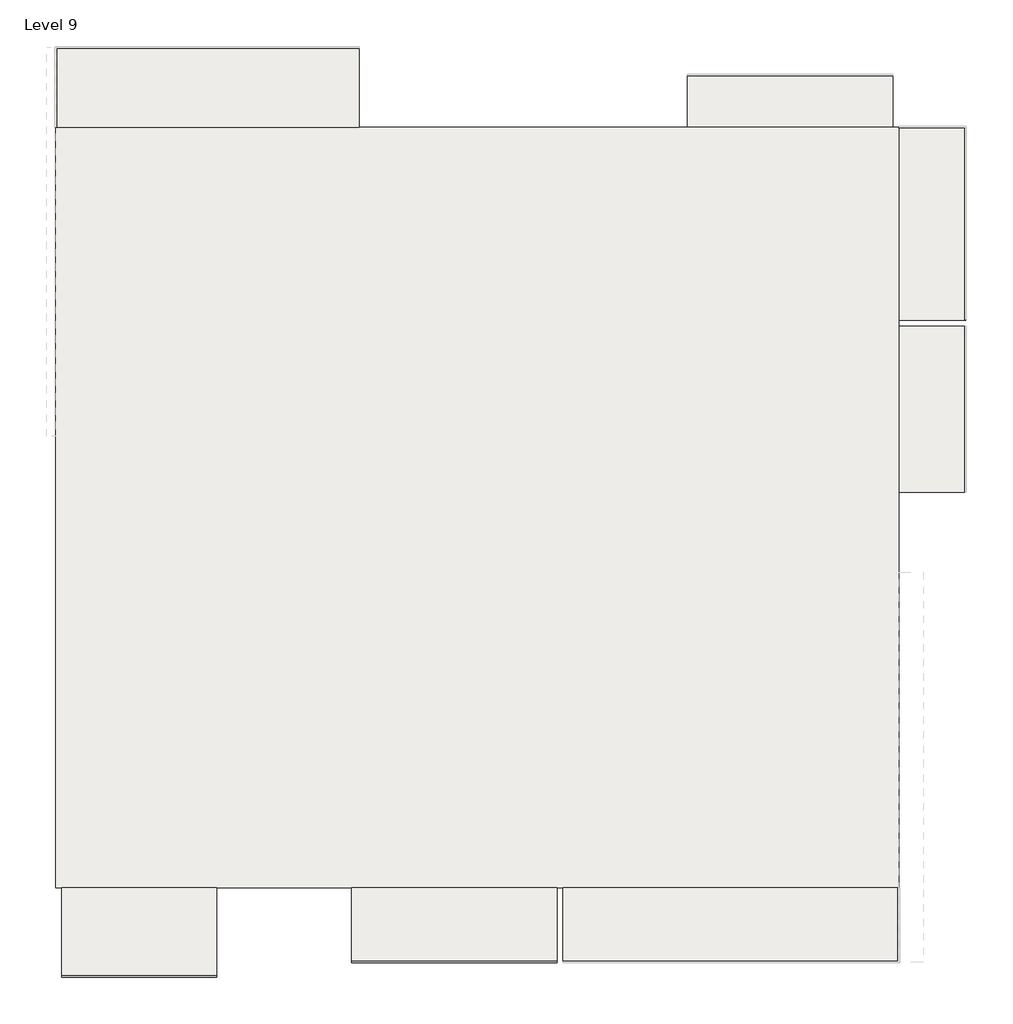
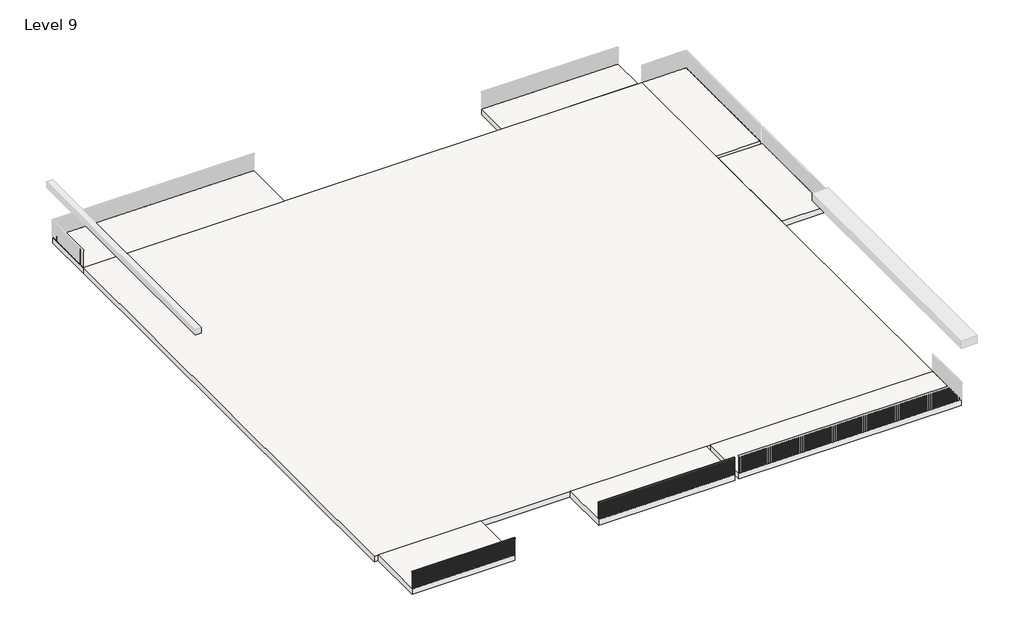
# One storey, part 1 of 5: 8 slabs, 2 railings.
"""IFC4 building model written with IfcOpenShell, lengths in millimetres."""

from ifc_helpers import new_model, si_unit, frame, origin, place, context, project, spatial, polyline, outline, extrude, element, save

model = new_model("IFC4")

# Units and contexts
model_context = context("Model", 3, world=origin())
ifc_project = project(units=[si_unit("LENGTHUNIT", "METRE", prefix="MILLI")], contexts=[model_context])

# Site, building, storey
site = spatial("IfcSite", under=ifc_project)
building = spatial("IfcBuilding", under=site)
storey = spatial("IfcBuildingStorey", under=building, Name="Level 9", Elevation=9448.8)

# Railings
placement = place(None, origin())
element("IfcRailing", 1, ObjectType="Handrail - Rectangular", at=placement, inside=storey, context=model_context, shape_type="SweptSolid", body=[
    extrude(outline(polyline([(-13630.2638778, -13399.9762475), (-13630.2638778, -13349.1762475), (-8499.4638778, -13349.1762475), (-8499.4638778, -13399.9762475), (-13630.2638778, -13399.9762475)])), frame((0.0, 0.0, 10312.4), z_axis=(0.0, 0.0, 1.0), x_axis=(1.0, 0.0, 0.0)), (0.0, 0.0, 1.0), 50.8),
    extrude(outline(polyline([(-8559.7888778, -13384.1012475), (-8559.7888778, -13365.0512475), (-8540.7388778, -13365.0512475), (-8540.7388778, -13384.1012475), (-8559.7888778, -13384.1012475)])), frame((0.0, 0.0, 9448.8), z_axis=(0.0, 0.0, 1.0), x_axis=(1.0, 0.0, 0.0)), (0.0, 0.0, 1.0), 863.6),
    extrude(outline(polyline([(-8661.3888778, -13384.1012475), (-8661.3888778, -13365.0512475), (-8642.3388778, -13365.0512475), (-8642.3388778, -13384.1012475), (-8661.3888778, -13384.1012475)])), frame((0.0, 0.0, 9448.8), z_axis=(0.0, 0.0, 1.0), x_axis=(1.0, 0.0, 0.0)), (0.0, 0.0, 1.0), 863.6),
    extrude(outline(polyline([(-8762.9888778, -13384.1012475), (-8762.9888778, -13365.0512475), (-8743.9388778, -13365.0512475), (-8743.9388778, -13384.1012475), (-8762.9888778, -13384.1012475)])), frame((0.0, 0.0, 9448.8), z_axis=(0.0, 0.0, 1.0), x_axis=(1.0, 0.0, 0.0)), (0.0, 0.0, 1.0), 863.6),
    extrude(outline(polyline([(-8864.5888778, -13384.1012475), (-8864.5888778, -13365.0512475), (-8845.5388778, -13365.0512475), (-8845.5388778, -13384.1012475), (-8864.5888778, -13384.1012475)])), frame((0.0, 0.0, 9448.8), z_axis=(0.0, 0.0, 1.0), x_axis=(1.0, 0.0, 0.0)), (0.0, 0.0, 1.0), 863.6),
    extrude(outline(polyline([(-8966.1888778, -13384.1012475), (-8966.1888778, -13365.0512475), (-8947.1388778, -13365.0512475), (-8947.1388778, -13384.1012475), (-8966.1888778, -13384.1012475)])), frame((0.0, 0.0, 9448.8), z_axis=(0.0, 0.0, 1.0), x_axis=(1.0, 0.0, 0.0)), (0.0, 0.0, 1.0), 863.6),
    extrude(outline(polyline([(-9067.7888778, -13384.1012475), (-9067.7888778, -13365.0512475), (-9048.7388778, -13365.0512475), (-9048.7388778, -13384.1012475), (-9067.7888778, -13384.1012475)])), frame((0.0, 0.0, 9448.8), z_axis=(0.0, 0.0, 1.0), x_axis=(1.0, 0.0, 0.0)), (0.0, 0.0, 1.0), 863.6),
    extrude(outline(polyline([(-9169.3888778, -13384.1012475), (-9169.3888778, -13365.0512475), (-9150.3388778, -13365.0512475), (-9150.3388778, -13384.1012475), (-9169.3888778, -13384.1012475)])), frame((0.0, 0.0, 9448.8), z_axis=(0.0, 0.0, 1.0), x_axis=(1.0, 0.0, 0.0)), (0.0, 0.0, 1.0), 863.6),
    extrude(outline(polyline([(-9270.9888778, -13384.1012475), (-9270.9888778, -13365.0512475), (-9251.9388778, -13365.0512475), (-9251.9388778, -13384.1012475), (-9270.9888778, -13384.1012475)])), frame((0.0, 0.0, 9448.8), z_axis=(0.0, 0.0, 1.0), x_axis=(1.0, 0.0, 0.0)), (0.0, 0.0, 1.0), 863.6),
    extrude(outline(polyline([(-9372.5888778, -13384.1012475), (-9372.5888778, -13365.0512475), (-9353.5388778, -13365.0512475), (-9353.5388778, -13384.1012475), (-9372.5888778, -13384.1012475)])), frame((0.0, 0.0, 9448.8), z_axis=(0.0, 0.0, 1.0), x_axis=(1.0, 0.0, 0.0)), (0.0, 0.0, 1.0), 863.6),
    extrude(outline(polyline([(-9474.1888778, -13384.1012475), (-9474.1888778, -13365.0512475), (-9455.1388778, -13365.0512475), (-9455.1388778, -13384.1012475), (-9474.1888778, -13384.1012475)])), frame((0.0, 0.0, 9448.8), z_axis=(0.0, 0.0, 1.0), x_axis=(1.0, 0.0, 0.0)), (0.0, 0.0, 1.0), 863.6),
    extrude(outline(polyline([(-9575.7888778, -13384.1012475), (-9575.7888778, -13365.0512475), (-9556.7388778, -13365.0512475), (-9556.7388778, -13384.1012475), (-9575.7888778, -13384.1012475)])), frame((0.0, 0.0, 9448.8), z_axis=(0.0, 0.0, 1.0), x_axis=(1.0, 0.0, 0.0)), (0.0, 0.0, 1.0), 863.6),
    extrude(outline(polyline([(-9677.3888778, -13384.1012475), (-9677.3888778, -13365.0512475), (-9658.3388778, -13365.0512475), (-9658.3388778, -13384.1012475), (-9677.3888778, -13384.1012475)])), frame((0.0, 0.0, 9448.8), z_axis=(0.0, 0.0, 1.0), x_axis=(1.0, 0.0, 0.0)), (0.0, 0.0, 1.0), 863.6),
    extrude(outline(polyline([(-9778.9888778, -13384.1012475), (-9778.9888778, -13365.0512475), (-9759.9388778, -13365.0512475), (-9759.9388778, -13384.1012475), (-9778.9888778, -13384.1012475)])), frame((0.0, 0.0, 9448.8), z_axis=(0.0, 0.0, 1.0), x_axis=(1.0, 0.0, 0.0)), (0.0, 0.0, 1.0), 863.6),
    extrude(outline(polyline([(-9880.5888778, -13384.1012475), (-9880.5888778, -13365.0512475), (-9861.5388778, -13365.0512475), (-9861.5388778, -13384.1012475), (-9880.5888778, -13384.1012475)])), frame((0.0, 0.0, 9448.8), z_axis=(0.0, 0.0, 1.0), x_axis=(1.0, 0.0, 0.0)), (0.0, 0.0, 1.0), 863.6),
    extrude(outline(polyline([(-9982.1888778, -13384.1012475), (-9982.1888778, -13365.0512475), (-9963.1388778, -13365.0512475), (-9963.1388778, -13384.1012475), (-9982.1888778, -13384.1012475)])), frame((0.0, 0.0, 9448.8), z_axis=(0.0, 0.0, 1.0), x_axis=(1.0, 0.0, 0.0)), (0.0, 0.0, 1.0), 863.6),
    extrude(outline(polyline([(-10083.7888778, -13384.1012475), (-10083.7888778, -13365.0512475), (-10064.7388778, -13365.0512475), (-10064.7388778, -13384.1012475), (-10083.7888778, -13384.1012475)])), frame((0.0, 0.0, 9448.8), z_axis=(0.0, 0.0, 1.0), x_axis=(1.0, 0.0, 0.0)), (0.0, 0.0, 1.0), 863.6),
    extrude(outline(polyline([(-10185.3888778, -13384.1012475), (-10185.3888778, -13365.0512475), (-10166.3388778, -13365.0512475), (-10166.3388778, -13384.1012475), (-10185.3888778, -13384.1012475)])), frame((0.0, 0.0, 9448.8), z_axis=(0.0, 0.0, 1.0), x_axis=(1.0, 0.0, 0.0)), (0.0, 0.0, 1.0), 863.6),
    extrude(outline(polyline([(-10286.9888778, -13384.1012475), (-10286.9888778, -13365.0512475), (-10267.9388778, -13365.0512475), (-10267.9388778, -13384.1012475), (-10286.9888778, -13384.1012475)])), frame((0.0, 0.0, 9448.8), z_axis=(0.0, 0.0, 1.0), x_axis=(1.0, 0.0, 0.0)), (0.0, 0.0, 1.0), 863.6),
    extrude(outline(polyline([(-10388.5888778, -13384.1012475), (-10388.5888778, -13365.0512475), (-10369.5388778, -13365.0512475), (-10369.5388778, -13384.1012475), (-10388.5888778, -13384.1012475)])), frame((0.0, 0.0, 9448.8), z_axis=(0.0, 0.0, 1.0), x_axis=(1.0, 0.0, 0.0)), (0.0, 0.0, 1.0), 863.6),
    extrude(outline(polyline([(-10490.1888778, -13384.1012475), (-10490.1888778, -13365.0512475), (-10471.1388778, -13365.0512475), (-10471.1388778, -13384.1012475), (-10490.1888778, -13384.1012475)])), frame((0.0, 0.0, 9448.8), z_axis=(0.0, 0.0, 1.0), x_axis=(1.0, 0.0, 0.0)), (0.0, 0.0, 1.0), 863.6),
    extrude(outline(polyline([(-10591.7888778, -13384.1012475), (-10591.7888778, -13365.0512475), (-10572.7388778, -13365.0512475), (-10572.7388778, -13384.1012475), (-10591.7888778, -13384.1012475)])), frame((0.0, 0.0, 9448.8), z_axis=(0.0, 0.0, 1.0), x_axis=(1.0, 0.0, 0.0)), (0.0, 0.0, 1.0), 863.6),
    extrude(outline(polyline([(-10693.3888778, -13384.1012475), (-10693.3888778, -13365.0512475), (-10674.3388778, -13365.0512475), (-10674.3388778, -13384.1012475), (-10693.3888778, -13384.1012475)])), frame((0.0, 0.0, 9448.8), z_axis=(0.0, 0.0, 1.0), x_axis=(1.0, 0.0, 0.0)), (0.0, 0.0, 1.0), 863.6),
    extrude(outline(polyline([(-10794.9888778, -13384.1012475), (-10794.9888778, -13365.0512475), (-10775.9388778, -13365.0512475), (-10775.9388778, -13384.1012475), (-10794.9888778, -13384.1012475)])), frame((0.0, 0.0, 9448.8), z_axis=(0.0, 0.0, 1.0), x_axis=(1.0, 0.0, 0.0)), (0.0, 0.0, 1.0), 863.6),
    extrude(outline(polyline([(-10896.5888778, -13384.1012475), (-10896.5888778, -13365.0512475), (-10877.5388778, -13365.0512475), (-10877.5388778, -13384.1012475), (-10896.5888778, -13384.1012475)])), frame((0.0, 0.0, 9448.8), z_axis=(0.0, 0.0, 1.0), x_axis=(1.0, 0.0, 0.0)), (0.0, 0.0, 1.0), 863.6),
    extrude(outline(polyline([(-10998.1888778, -13384.1012475), (-10998.1888778, -13365.0512475), (-10979.1388778, -13365.0512475), (-10979.1388778, -13384.1012475), (-10998.1888778, -13384.1012475)])), frame((0.0, 0.0, 9448.8), z_axis=(0.0, 0.0, 1.0), x_axis=(1.0, 0.0, 0.0)), (0.0, 0.0, 1.0), 863.6),
    extrude(outline(polyline([(-11099.7888778, -13384.1012475), (-11099.7888778, -13365.0512475), (-11080.7388778, -13365.0512475), (-11080.7388778, -13384.1012475), (-11099.7888778, -13384.1012475)])), frame((0.0, 0.0, 9448.8), z_axis=(0.0, 0.0, 1.0), x_axis=(1.0, 0.0, 0.0)), (0.0, 0.0, 1.0), 863.6),
    extrude(outline(polyline([(-11201.3888778, -13384.1012475), (-11201.3888778, -13365.0512475), (-11182.3388778, -13365.0512475), (-11182.3388778, -13384.1012475), (-11201.3888778, -13384.1012475)])), frame((0.0, 0.0, 9448.8), z_axis=(0.0, 0.0, 1.0), x_axis=(1.0, 0.0, 0.0)), (0.0, 0.0, 1.0), 863.6),
    extrude(outline(polyline([(-11302.9888778, -13384.1012475), (-11302.9888778, -13365.0512475), (-11283.9388778, -13365.0512475), (-11283.9388778, -13384.1012475), (-11302.9888778, -13384.1012475)])), frame((0.0, 0.0, 9448.8), z_axis=(0.0, 0.0, 1.0), x_axis=(1.0, 0.0, 0.0)), (0.0, 0.0, 1.0), 863.6),
    extrude(outline(polyline([(-11404.5888778, -13384.1012475), (-11404.5888778, -13365.0512475), (-11385.5388778, -13365.0512475), (-11385.5388778, -13384.1012475), (-11404.5888778, -13384.1012475)])), frame((0.0, 0.0, 9448.8), z_axis=(0.0, 0.0, 1.0), x_axis=(1.0, 0.0, 0.0)), (0.0, 0.0, 1.0), 863.6),
    extrude(outline(polyline([(-11506.1888778, -13384.1012475), (-11506.1888778, -13365.0512475), (-11487.1388778, -13365.0512475), (-11487.1388778, -13384.1012475), (-11506.1888778, -13384.1012475)])), frame((0.0, 0.0, 9448.8), z_axis=(0.0, 0.0, 1.0), x_axis=(1.0, 0.0, 0.0)), (0.0, 0.0, 1.0), 863.6),
    extrude(outline(polyline([(-11607.7888778, -13384.1012475), (-11607.7888778, -13365.0512475), (-11588.7388778, -13365.0512475), (-11588.7388778, -13384.1012475), (-11607.7888778, -13384.1012475)])), frame((0.0, 0.0, 9448.8), z_axis=(0.0, 0.0, 1.0), x_axis=(1.0, 0.0, 0.0)), (0.0, 0.0, 1.0), 863.6),
    extrude(outline(polyline([(-11709.3888778, -13384.1012475), (-11709.3888778, -13365.0512475), (-11690.3388778, -13365.0512475), (-11690.3388778, -13384.1012475), (-11709.3888778, -13384.1012475)])), frame((0.0, 0.0, 9448.8), z_axis=(0.0, 0.0, 1.0), x_axis=(1.0, 0.0, 0.0)), (0.0, 0.0, 1.0), 863.6),
    extrude(outline(polyline([(-11810.9888778, -13384.1012475), (-11810.9888778, -13365.0512475), (-11791.9388778, -13365.0512475), (-11791.9388778, -13384.1012475), (-11810.9888778, -13384.1012475)])), frame((0.0, 0.0, 9448.8), z_axis=(0.0, 0.0, 1.0), x_axis=(1.0, 0.0, 0.0)), (0.0, 0.0, 1.0), 863.6),
    extrude(outline(polyline([(-11912.5888778, -13384.1012475), (-11912.5888778, -13365.0512475), (-11893.5388778, -13365.0512475), (-11893.5388778, -13384.1012475), (-11912.5888778, -13384.1012475)])), frame((0.0, 0.0, 9448.8), z_axis=(0.0, 0.0, 1.0), x_axis=(1.0, 0.0, 0.0)), (0.0, 0.0, 1.0), 863.6),
    extrude(outline(polyline([(-12014.1888778, -13384.1012475), (-12014.1888778, -13365.0512475), (-11995.1388778, -13365.0512475), (-11995.1388778, -13384.1012475), (-12014.1888778, -13384.1012475)])), frame((0.0, 0.0, 9448.8), z_axis=(0.0, 0.0, 1.0), x_axis=(1.0, 0.0, 0.0)), (0.0, 0.0, 1.0), 863.6),
    extrude(outline(polyline([(-12115.7888778, -13384.1012475), (-12115.7888778, -13365.0512475), (-12096.7388778, -13365.0512475), (-12096.7388778, -13384.1012475), (-12115.7888778, -13384.1012475)])), frame((0.0, 0.0, 9448.8), z_axis=(0.0, 0.0, 1.0), x_axis=(1.0, 0.0, 0.0)), (0.0, 0.0, 1.0), 863.6),
    extrude(outline(polyline([(-12217.3888778, -13384.1012475), (-12217.3888778, -13365.0512475), (-12198.3388778, -13365.0512475), (-12198.3388778, -13384.1012475), (-12217.3888778, -13384.1012475)])), frame((0.0, 0.0, 9448.8), z_axis=(0.0, 0.0, 1.0), x_axis=(1.0, 0.0, 0.0)), (0.0, 0.0, 1.0), 863.6),
    extrude(outline(polyline([(-12318.9888778, -13384.1012475), (-12318.9888778, -13365.0512475), (-12299.9388778, -13365.0512475), (-12299.9388778, -13384.1012475), (-12318.9888778, -13384.1012475)])), frame((0.0, 0.0, 9448.8), z_axis=(0.0, 0.0, 1.0), x_axis=(1.0, 0.0, 0.0)), (0.0, 0.0, 1.0), 863.6),
    extrude(outline(polyline([(-12420.5888778, -13384.1012475), (-12420.5888778, -13365.0512475), (-12401.5388778, -13365.0512475), (-12401.5388778, -13384.1012475), (-12420.5888778, -13384.1012475)])), frame((0.0, 0.0, 9448.8), z_axis=(0.0, 0.0, 1.0), x_axis=(1.0, 0.0, 0.0)), (0.0, 0.0, 1.0), 863.6),
    extrude(outline(polyline([(-12522.1888778, -13384.1012475), (-12522.1888778, -13365.0512475), (-12503.1388778, -13365.0512475), (-12503.1388778, -13384.1012475), (-12522.1888778, -13384.1012475)])), frame((0.0, 0.0, 9448.8), z_axis=(0.0, 0.0, 1.0), x_axis=(1.0, 0.0, 0.0)), (0.0, 0.0, 1.0), 863.6),
    extrude(outline(polyline([(-12623.7888778, -13384.1012475), (-12623.7888778, -13365.0512475), (-12604.7388778, -13365.0512475), (-12604.7388778, -13384.1012475), (-12623.7888778, -13384.1012475)])), frame((0.0, 0.0, 9448.8), z_axis=(0.0, 0.0, 1.0), x_axis=(1.0, 0.0, 0.0)), (0.0, 0.0, 1.0), 863.6),
    extrude(outline(polyline([(-12725.3888778, -13384.1012475), (-12725.3888778, -13365.0512475), (-12706.3388778, -13365.0512475), (-12706.3388778, -13384.1012475), (-12725.3888778, -13384.1012475)])), frame((0.0, 0.0, 9448.8), z_axis=(0.0, 0.0, 1.0), x_axis=(1.0, 0.0, 0.0)), (0.0, 0.0, 1.0), 863.6),
    extrude(outline(polyline([(-12826.9888778, -13384.1012475), (-12826.9888778, -13365.0512475), (-12807.9388778, -13365.0512475), (-12807.9388778, -13384.1012475), (-12826.9888778, -13384.1012475)])), frame((0.0, 0.0, 9448.8), z_axis=(0.0, 0.0, 1.0), x_axis=(1.0, 0.0, 0.0)), (0.0, 0.0, 1.0), 863.6),
    extrude(outline(polyline([(-12928.5888778, -13384.1012475), (-12928.5888778, -13365.0512475), (-12909.5388778, -13365.0512475), (-12909.5388778, -13384.1012475), (-12928.5888778, -13384.1012475)])), frame((0.0, 0.0, 9448.8), z_axis=(0.0, 0.0, 1.0), x_axis=(1.0, 0.0, 0.0)), (0.0, 0.0, 1.0), 863.6),
    extrude(outline(polyline([(-13030.1888778, -13384.1012475), (-13030.1888778, -13365.0512475), (-13011.1388778, -13365.0512475), (-13011.1388778, -13384.1012475), (-13030.1888778, -13384.1012475)])), frame((0.0, 0.0, 9448.8), z_axis=(0.0, 0.0, 1.0), x_axis=(1.0, 0.0, 0.0)), (0.0, 0.0, 1.0), 863.6),
    extrude(outline(polyline([(-13131.7888778, -13384.1012475), (-13131.7888778, -13365.0512475), (-13112.7388778, -13365.0512475), (-13112.7388778, -13384.1012475), (-13131.7888778, -13384.1012475)])), frame((0.0, 0.0, 9448.8), z_axis=(0.0, 0.0, 1.0), x_axis=(1.0, 0.0, 0.0)), (0.0, 0.0, 1.0), 863.6),
    extrude(outline(polyline([(-13233.3888778, -13384.1012475), (-13233.3888778, -13365.0512475), (-13214.3388778, -13365.0512475), (-13214.3388778, -13384.1012475), (-13233.3888778, -13384.1012475)])), frame((0.0, 0.0, 9448.8), z_axis=(0.0, 0.0, 1.0), x_axis=(1.0, 0.0, 0.0)), (0.0, 0.0, 1.0), 863.6),
    extrude(outline(polyline([(-13334.9888778, -13384.1012475), (-13334.9888778, -13365.0512475), (-13315.9388778, -13365.0512475), (-13315.9388778, -13384.1012475), (-13334.9888778, -13384.1012475)])), frame((0.0, 0.0, 9448.8), z_axis=(0.0, 0.0, 1.0), x_axis=(1.0, 0.0, 0.0)), (0.0, 0.0, 1.0), 863.6),
    extrude(outline(polyline([(-13436.5888778, -13384.1012475), (-13436.5888778, -13365.0512475), (-13417.5388778, -13365.0512475), (-13417.5388778, -13384.1012475), (-13436.5888778, -13384.1012475)])), frame((0.0, 0.0, 9448.8), z_axis=(0.0, 0.0, 1.0), x_axis=(1.0, 0.0, 0.0)), (0.0, 0.0, 1.0), 863.6),
    extrude(outline(polyline([(-13538.1888778, -13384.1012475), (-13538.1888778, -13365.0512475), (-13519.1388778, -13365.0512475), (-13519.1388778, -13384.1012475), (-13538.1888778, -13384.1012475)])), frame((0.0, 0.0, 9448.8), z_axis=(0.0, 0.0, 1.0), x_axis=(1.0, 0.0, 0.0)), (0.0, 0.0, 1.0), 863.6),
    extrude(outline(polyline([(-8518.5138778, -13384.1012475), (-8518.5138778, -13365.0512475), (-8499.4638778, -13365.0512475), (-8499.4638778, -13384.1012475), (-8518.5138778, -13384.1012475)])), frame((0.0, 0.0, 9448.8), z_axis=(0.0, 0.0, 1.0), x_axis=(1.0, 0.0, 0.0)), (0.0, 0.0, 1.0), 863.6),
    extrude(outline(polyline([(-13630.2638778, -13384.1012475), (-13630.2638778, -13365.0512475), (-13611.2138778, -13365.0512475), (-13611.2138778, -13384.1012475), (-13630.2638778, -13384.1012475)])), frame((0.0, 0.0, 9448.8), z_axis=(0.0, 0.0, 1.0), x_axis=(1.0, 0.0, 0.0)), (0.0, 0.0, 1.0), 863.6),
])
element("IfcRailing", 2, ObjectType="Handrail - Rectangular", at=placement, inside=storey, context=model_context, shape_type="SweptSolid", body=[
    extrude(outline(polyline([(-4029.0638778, -12911.7749501), (-4029.0638778, -12860.9749501), (2778.1361222, -12860.9749501), (2778.1361222, -12911.7749501), (-4029.0638778, -12911.7749501)])), frame((0.0, 0.0, 10312.4), z_axis=(0.0, 0.0, 1.0), x_axis=(1.0, 0.0, 0.0)), (0.0, 0.0, 1.0), 50.8),
    extrude(outline(polyline([(2667.0111222, -12895.8999501), (2667.0111222, -12876.8499501), (2686.0611222, -12876.8499501), (2686.0611222, -12895.8999501), (2667.0111222, -12895.8999501)])), frame((0.0, 0.0, 9448.8), z_axis=(0.0, 0.0, 1.0), x_axis=(1.0, 0.0, 0.0)), (0.0, 0.0, 1.0), 863.6),
    extrude(outline(polyline([(2565.4111222, -12895.8999501), (2565.4111222, -12876.8499501), (2584.4611222, -12876.8499501), (2584.4611222, -12895.8999501), (2565.4111222, -12895.8999501)])), frame((0.0, 0.0, 9448.8), z_axis=(0.0, 0.0, 1.0), x_axis=(1.0, 0.0, 0.0)), (0.0, 0.0, 1.0), 863.6),
    extrude(outline(polyline([(2463.8111222, -12895.8999501), (2463.8111222, -12876.8499501), (2482.8611222, -12876.8499501), (2482.8611222, -12895.8999501), (2463.8111222, -12895.8999501)])), frame((0.0, 0.0, 9448.8), z_axis=(0.0, 0.0, 1.0), x_axis=(1.0, 0.0, 0.0)), (0.0, 0.0, 1.0), 863.6),
    extrude(outline(polyline([(2362.2111222, -12895.8999501), (2362.2111222, -12876.8499501), (2381.2611222, -12876.8499501), (2381.2611222, -12895.8999501), (2362.2111222, -12895.8999501)])), frame((0.0, 0.0, 9448.8), z_axis=(0.0, 0.0, 1.0), x_axis=(1.0, 0.0, 0.0)), (0.0, 0.0, 1.0), 863.6),
    extrude(outline(polyline([(2260.6111222, -12895.8999501), (2260.6111222, -12876.8499501), (2279.6611222, -12876.8499501), (2279.6611222, -12895.8999501), (2260.6111222, -12895.8999501)])), frame((0.0, 0.0, 9448.8), z_axis=(0.0, 0.0, 1.0), x_axis=(1.0, 0.0, 0.0)), (0.0, 0.0, 1.0), 863.6),
    extrude(outline(polyline([(2159.0111222, -12895.8999501), (2159.0111222, -12876.8499501), (2178.0611222, -12876.8499501), (2178.0611222, -12895.8999501), (2159.0111222, -12895.8999501)])), frame((0.0, 0.0, 9448.8), z_axis=(0.0, 0.0, 1.0), x_axis=(1.0, 0.0, 0.0)), (0.0, 0.0, 1.0), 863.6),
    extrude(outline(polyline([(2057.4111222, -12895.8999501), (2057.4111222, -12876.8499501), (2076.4611222, -12876.8499501), (2076.4611222, -12895.8999501), (2057.4111222, -12895.8999501)])), frame((0.0, 0.0, 9448.8), z_axis=(0.0, 0.0, 1.0), x_axis=(1.0, 0.0, 0.0)), (0.0, 0.0, 1.0), 863.6),
    extrude(outline(polyline([(1955.8111222, -12895.8999501), (1955.8111222, -12876.8499501), (1974.8611222, -12876.8499501), (1974.8611222, -12895.8999501), (1955.8111222, -12895.8999501)])), frame((0.0, 0.0, 9448.8), z_axis=(0.0, 0.0, 1.0), x_axis=(1.0, 0.0, 0.0)), (0.0, 0.0, 1.0), 863.6),
    extrude(outline(polyline([(1854.2111222, -12895.8999501), (1854.2111222, -12876.8499501), (1873.2611222, -12876.8499501), (1873.2611222, -12895.8999501), (1854.2111222, -12895.8999501)])), frame((0.0, 0.0, 9448.8), z_axis=(0.0, 0.0, 1.0), x_axis=(1.0, 0.0, 0.0)), (0.0, 0.0, 1.0), 863.6),
    extrude(outline(polyline([(1752.6111222, -12895.8999501), (1752.6111222, -12876.8499501), (1771.6611222, -12876.8499501), (1771.6611222, -12895.8999501), (1752.6111222, -12895.8999501)])), frame((0.0, 0.0, 9448.8), z_axis=(0.0, 0.0, 1.0), x_axis=(1.0, 0.0, 0.0)), (0.0, 0.0, 1.0), 863.6),
    extrude(outline(polyline([(1651.0111222, -12895.8999501), (1651.0111222, -12876.8499501), (1670.0611222, -12876.8499501), (1670.0611222, -12895.8999501), (1651.0111222, -12895.8999501)])), frame((0.0, 0.0, 9448.8), z_axis=(0.0, 0.0, 1.0), x_axis=(1.0, 0.0, 0.0)), (0.0, 0.0, 1.0), 863.6),
    extrude(outline(polyline([(1549.4111222, -12895.8999501), (1549.4111222, -12876.8499501), (1568.4611222, -12876.8499501), (1568.4611222, -12895.8999501), (1549.4111222, -12895.8999501)])), frame((0.0, 0.0, 9448.8), z_axis=(0.0, 0.0, 1.0), x_axis=(1.0, 0.0, 0.0)), (0.0, 0.0, 1.0), 863.6),
    extrude(outline(polyline([(1447.8111222, -12895.8999501), (1447.8111222, -12876.8499501), (1466.8611222, -12876.8499501), (1466.8611222, -12895.8999501), (1447.8111222, -12895.8999501)])), frame((0.0, 0.0, 9448.8), z_axis=(0.0, 0.0, 1.0), x_axis=(1.0, 0.0, 0.0)), (0.0, 0.0, 1.0), 863.6),
    extrude(outline(polyline([(1346.2111222, -12895.8999501), (1346.2111222, -12876.8499501), (1365.2611222, -12876.8499501), (1365.2611222, -12895.8999501), (1346.2111222, -12895.8999501)])), frame((0.0, 0.0, 9448.8), z_axis=(0.0, 0.0, 1.0), x_axis=(1.0, 0.0, 0.0)), (0.0, 0.0, 1.0), 863.6),
    extrude(outline(polyline([(1244.6111222, -12895.8999501), (1244.6111222, -12876.8499501), (1263.6611222, -12876.8499501), (1263.6611222, -12895.8999501), (1244.6111222, -12895.8999501)])), frame((0.0, 0.0, 9448.8), z_axis=(0.0, 0.0, 1.0), x_axis=(1.0, 0.0, 0.0)), (0.0, 0.0, 1.0), 863.6),
    extrude(outline(polyline([(1143.0111222, -12895.8999501), (1143.0111222, -12876.8499501), (1162.0611222, -12876.8499501), (1162.0611222, -12895.8999501), (1143.0111222, -12895.8999501)])), frame((0.0, 0.0, 9448.8), z_axis=(0.0, 0.0, 1.0), x_axis=(1.0, 0.0, 0.0)), (0.0, 0.0, 1.0), 863.6),
    extrude(outline(polyline([(1041.4111222, -12895.8999501), (1041.4111222, -12876.8499501), (1060.4611222, -12876.8499501), (1060.4611222, -12895.8999501), (1041.4111222, -12895.8999501)])), frame((0.0, 0.0, 9448.8), z_axis=(0.0, 0.0, 1.0), x_axis=(1.0, 0.0, 0.0)), (0.0, 0.0, 1.0), 863.6),
    extrude(outline(polyline([(939.8111222, -12895.8999501), (939.8111222, -12876.8499501), (958.8611222, -12876.8499501), (958.8611222, -12895.8999501), (939.8111222, -12895.8999501)])), frame((0.0, 0.0, 9448.8), z_axis=(0.0, 0.0, 1.0), x_axis=(1.0, 0.0, 0.0)), (0.0, 0.0, 1.0), 863.6),
    extrude(outline(polyline([(838.2111222, -12895.8999501), (838.2111222, -12876.8499501), (857.2611222, -12876.8499501), (857.2611222, -12895.8999501), (838.2111222, -12895.8999501)])), frame((0.0, 0.0, 9448.8), z_axis=(0.0, 0.0, 1.0), x_axis=(1.0, 0.0, 0.0)), (0.0, 0.0, 1.0), 863.6),
    extrude(outline(polyline([(736.6111222, -12895.8999501), (736.6111222, -12876.8499501), (755.6611222, -12876.8499501), (755.6611222, -12895.8999501), (736.6111222, -12895.8999501)])), frame((0.0, 0.0, 9448.8), z_axis=(0.0, 0.0, 1.0), x_axis=(1.0, 0.0, 0.0)), (0.0, 0.0, 1.0), 863.6),
    extrude(outline(polyline([(635.0111222, -12895.8999501), (635.0111222, -12876.8499501), (654.0611222, -12876.8499501), (654.0611222, -12895.8999501), (635.0111222, -12895.8999501)])), frame((0.0, 0.0, 9448.8), z_axis=(0.0, 0.0, 1.0), x_axis=(1.0, 0.0, 0.0)), (0.0, 0.0, 1.0), 863.6),
    extrude(outline(polyline([(533.4111222, -12895.8999501), (533.4111222, -12876.8499501), (552.4611222, -12876.8499501), (552.4611222, -12895.8999501), (533.4111222, -12895.8999501)])), frame((0.0, 0.0, 9448.8), z_axis=(0.0, 0.0, 1.0), x_axis=(1.0, 0.0, 0.0)), (0.0, 0.0, 1.0), 863.6),
    extrude(outline(polyline([(431.8111222, -12895.8999501), (431.8111222, -12876.8499501), (450.8611222, -12876.8499501), (450.8611222, -12895.8999501), (431.8111222, -12895.8999501)])), frame((0.0, 0.0, 9448.8), z_axis=(0.0, 0.0, 1.0), x_axis=(1.0, 0.0, 0.0)), (0.0, 0.0, 1.0), 863.6),
    extrude(outline(polyline([(330.2111222, -12895.8999501), (330.2111222, -12876.8499501), (349.2611222, -12876.8499501), (349.2611222, -12895.8999501), (330.2111222, -12895.8999501)])), frame((0.0, 0.0, 9448.8), z_axis=(0.0, 0.0, 1.0), x_axis=(1.0, 0.0, 0.0)), (0.0, 0.0, 1.0), 863.6),
    extrude(outline(polyline([(228.6111222, -12895.8999501), (228.6111222, -12876.8499501), (247.6611222, -12876.8499501), (247.6611222, -12895.8999501), (228.6111222, -12895.8999501)])), frame((0.0, 0.0, 9448.8), z_axis=(0.0, 0.0, 1.0), x_axis=(1.0, 0.0, 0.0)), (0.0, 0.0, 1.0), 863.6),
    extrude(outline(polyline([(127.0111222, -12895.8999501), (127.0111222, -12876.8499501), (146.0611222, -12876.8499501), (146.0611222, -12895.8999501), (127.0111222, -12895.8999501)])), frame((0.0, 0.0, 9448.8), z_axis=(0.0, 0.0, 1.0), x_axis=(1.0, 0.0, 0.0)), (0.0, 0.0, 1.0), 863.6),
    extrude(outline(polyline([(25.4111222, -12895.8999501), (25.4111222, -12876.8499501), (44.4611222, -12876.8499501), (44.4611222, -12895.8999501), (25.4111222, -12895.8999501)])), frame((0.0, 0.0, 9448.8), z_axis=(0.0, 0.0, 1.0), x_axis=(1.0, 0.0, 0.0)), (0.0, 0.0, 1.0), 863.6),
    extrude(outline(polyline([(-76.1888778, -12895.8999501), (-76.1888778, -12876.8499501), (-57.1388778, -12876.8499501), (-57.1388778, -12895.8999501), (-76.1888778, -12895.8999501)])), frame((0.0, 0.0, 9448.8), z_axis=(0.0, 0.0, 1.0), x_axis=(1.0, 0.0, 0.0)), (0.0, 0.0, 1.0), 863.6),
    extrude(outline(polyline([(-177.7888778, -12895.8999501), (-177.7888778, -12876.8499501), (-158.7388778, -12876.8499501), (-158.7388778, -12895.8999501), (-177.7888778, -12895.8999501)])), frame((0.0, 0.0, 9448.8), z_axis=(0.0, 0.0, 1.0), x_axis=(1.0, 0.0, 0.0)), (0.0, 0.0, 1.0), 863.6),
    extrude(outline(polyline([(-279.3888778, -12895.8999501), (-279.3888778, -12876.8499501), (-260.3388778, -12876.8499501), (-260.3388778, -12895.8999501), (-279.3888778, -12895.8999501)])), frame((0.0, 0.0, 9448.8), z_axis=(0.0, 0.0, 1.0), x_axis=(1.0, 0.0, 0.0)), (0.0, 0.0, 1.0), 863.6),
    extrude(outline(polyline([(-380.9888778, -12895.8999501), (-380.9888778, -12876.8499501), (-361.9388778, -12876.8499501), (-361.9388778, -12895.8999501), (-380.9888778, -12895.8999501)])), frame((0.0, 0.0, 9448.8), z_axis=(0.0, 0.0, 1.0), x_axis=(1.0, 0.0, 0.0)), (0.0, 0.0, 1.0), 863.6),
    extrude(outline(polyline([(-482.5888778, -12895.8999501), (-482.5888778, -12876.8499501), (-463.5388778, -12876.8499501), (-463.5388778, -12895.8999501), (-482.5888778, -12895.8999501)])), frame((0.0, 0.0, 9448.8), z_axis=(0.0, 0.0, 1.0), x_axis=(1.0, 0.0, 0.0)), (0.0, 0.0, 1.0), 863.6),
    extrude(outline(polyline([(-584.1888778, -12895.8999501), (-584.1888778, -12876.8499501), (-565.1388778, -12876.8499501), (-565.1388778, -12895.8999501), (-584.1888778, -12895.8999501)])), frame((0.0, 0.0, 9448.8), z_axis=(0.0, 0.0, 1.0), x_axis=(1.0, 0.0, 0.0)), (0.0, 0.0, 1.0), 863.6),
    extrude(outline(polyline([(-685.7888778, -12895.8999501), (-685.7888778, -12876.8499501), (-666.7388778, -12876.8499501), (-666.7388778, -12895.8999501), (-685.7888778, -12895.8999501)])), frame((0.0, 0.0, 9448.8), z_axis=(0.0, 0.0, 1.0), x_axis=(1.0, 0.0, 0.0)), (0.0, 0.0, 1.0), 863.6),
    extrude(outline(polyline([(-787.3888778, -12895.8999501), (-787.3888778, -12876.8499501), (-768.3388778, -12876.8499501), (-768.3388778, -12895.8999501), (-787.3888778, -12895.8999501)])), frame((0.0, 0.0, 9448.8), z_axis=(0.0, 0.0, 1.0), x_axis=(1.0, 0.0, 0.0)), (0.0, 0.0, 1.0), 863.6),
    extrude(outline(polyline([(-888.9888778, -12895.8999501), (-888.9888778, -12876.8499501), (-869.9388778, -12876.8499501), (-869.9388778, -12895.8999501), (-888.9888778, -12895.8999501)])), frame((0.0, 0.0, 9448.8), z_axis=(0.0, 0.0, 1.0), x_axis=(1.0, 0.0, 0.0)), (0.0, 0.0, 1.0), 863.6),
    extrude(outline(polyline([(-990.5888778, -12895.8999501), (-990.5888778, -12876.8499501), (-971.5388778, -12876.8499501), (-971.5388778, -12895.8999501), (-990.5888778, -12895.8999501)])), frame((0.0, 0.0, 9448.8), z_axis=(0.0, 0.0, 1.0), x_axis=(1.0, 0.0, 0.0)), (0.0, 0.0, 1.0), 863.6),
    extrude(outline(polyline([(-1092.1888778, -12895.8999501), (-1092.1888778, -12876.8499501), (-1073.1388778, -12876.8499501), (-1073.1388778, -12895.8999501), (-1092.1888778, -12895.8999501)])), frame((0.0, 0.0, 9448.8), z_axis=(0.0, 0.0, 1.0), x_axis=(1.0, 0.0, 0.0)), (0.0, 0.0, 1.0), 863.6),
    extrude(outline(polyline([(-1193.7888778, -12895.8999501), (-1193.7888778, -12876.8499501), (-1174.7388778, -12876.8499501), (-1174.7388778, -12895.8999501), (-1193.7888778, -12895.8999501)])), frame((0.0, 0.0, 9448.8), z_axis=(0.0, 0.0, 1.0), x_axis=(1.0, 0.0, 0.0)), (0.0, 0.0, 1.0), 863.6),
    extrude(outline(polyline([(-1295.3888778, -12895.8999501), (-1295.3888778, -12876.8499501), (-1276.3388778, -12876.8499501), (-1276.3388778, -12895.8999501), (-1295.3888778, -12895.8999501)])), frame((0.0, 0.0, 9448.8), z_axis=(0.0, 0.0, 1.0), x_axis=(1.0, 0.0, 0.0)), (0.0, 0.0, 1.0), 863.6),
    extrude(outline(polyline([(-1396.9888778, -12895.8999501), (-1396.9888778, -12876.8499501), (-1377.9388778, -12876.8499501), (-1377.9388778, -12895.8999501), (-1396.9888778, -12895.8999501)])), frame((0.0, 0.0, 9448.8), z_axis=(0.0, 0.0, 1.0), x_axis=(1.0, 0.0, 0.0)), (0.0, 0.0, 1.0), 863.6),
    extrude(outline(polyline([(-1498.5888778, -12895.8999501), (-1498.5888778, -12876.8499501), (-1479.5388778, -12876.8499501), (-1479.5388778, -12895.8999501), (-1498.5888778, -12895.8999501)])), frame((0.0, 0.0, 9448.8), z_axis=(0.0, 0.0, 1.0), x_axis=(1.0, 0.0, 0.0)), (0.0, 0.0, 1.0), 863.6),
    extrude(outline(polyline([(-1600.1888778, -12895.8999501), (-1600.1888778, -12876.8499501), (-1581.1388778, -12876.8499501), (-1581.1388778, -12895.8999501), (-1600.1888778, -12895.8999501)])), frame((0.0, 0.0, 9448.8), z_axis=(0.0, 0.0, 1.0), x_axis=(1.0, 0.0, 0.0)), (0.0, 0.0, 1.0), 863.6),
    extrude(outline(polyline([(-1701.7888778, -12895.8999501), (-1701.7888778, -12876.8499501), (-1682.7388778, -12876.8499501), (-1682.7388778, -12895.8999501), (-1701.7888778, -12895.8999501)])), frame((0.0, 0.0, 9448.8), z_axis=(0.0, 0.0, 1.0), x_axis=(1.0, 0.0, 0.0)), (0.0, 0.0, 1.0), 863.6),
    extrude(outline(polyline([(-1803.3888778, -12895.8999501), (-1803.3888778, -12876.8499501), (-1784.3388778, -12876.8499501), (-1784.3388778, -12895.8999501), (-1803.3888778, -12895.8999501)])), frame((0.0, 0.0, 9448.8), z_axis=(0.0, 0.0, 1.0), x_axis=(1.0, 0.0, 0.0)), (0.0, 0.0, 1.0), 863.6),
    extrude(outline(polyline([(-1904.9888778, -12895.8999501), (-1904.9888778, -12876.8499501), (-1885.9388778, -12876.8499501), (-1885.9388778, -12895.8999501), (-1904.9888778, -12895.8999501)])), frame((0.0, 0.0, 9448.8), z_axis=(0.0, 0.0, 1.0), x_axis=(1.0, 0.0, 0.0)), (0.0, 0.0, 1.0), 863.6),
    extrude(outline(polyline([(-2006.5888778, -12895.8999501), (-2006.5888778, -12876.8499501), (-1987.5388778, -12876.8499501), (-1987.5388778, -12895.8999501), (-2006.5888778, -12895.8999501)])), frame((0.0, 0.0, 9448.8), z_axis=(0.0, 0.0, 1.0), x_axis=(1.0, 0.0, 0.0)), (0.0, 0.0, 1.0), 863.6),
    extrude(outline(polyline([(-2108.1888778, -12895.8999501), (-2108.1888778, -12876.8499501), (-2089.1388778, -12876.8499501), (-2089.1388778, -12895.8999501), (-2108.1888778, -12895.8999501)])), frame((0.0, 0.0, 9448.8), z_axis=(0.0, 0.0, 1.0), x_axis=(1.0, 0.0, 0.0)), (0.0, 0.0, 1.0), 863.6),
    extrude(outline(polyline([(-2209.7888778, -12895.8999501), (-2209.7888778, -12876.8499501), (-2190.7388778, -12876.8499501), (-2190.7388778, -12895.8999501), (-2209.7888778, -12895.8999501)])), frame((0.0, 0.0, 9448.8), z_axis=(0.0, 0.0, 1.0), x_axis=(1.0, 0.0, 0.0)), (0.0, 0.0, 1.0), 863.6),
    extrude(outline(polyline([(-2311.3888778, -12895.8999501), (-2311.3888778, -12876.8499501), (-2292.3388778, -12876.8499501), (-2292.3388778, -12895.8999501), (-2311.3888778, -12895.8999501)])), frame((0.0, 0.0, 9448.8), z_axis=(0.0, 0.0, 1.0), x_axis=(1.0, 0.0, 0.0)), (0.0, 0.0, 1.0), 863.6),
    extrude(outline(polyline([(-2412.9888778, -12895.8999501), (-2412.9888778, -12876.8499501), (-2393.9388778, -12876.8499501), (-2393.9388778, -12895.8999501), (-2412.9888778, -12895.8999501)])), frame((0.0, 0.0, 9448.8), z_axis=(0.0, 0.0, 1.0), x_axis=(1.0, 0.0, 0.0)), (0.0, 0.0, 1.0), 863.6),
    extrude(outline(polyline([(-2514.5888778, -12895.8999501), (-2514.5888778, -12876.8499501), (-2495.5388778, -12876.8499501), (-2495.5388778, -12895.8999501), (-2514.5888778, -12895.8999501)])), frame((0.0, 0.0, 9448.8), z_axis=(0.0, 0.0, 1.0), x_axis=(1.0, 0.0, 0.0)), (0.0, 0.0, 1.0), 863.6),
    extrude(outline(polyline([(-2616.1888778, -12895.8999501), (-2616.1888778, -12876.8499501), (-2597.1388778, -12876.8499501), (-2597.1388778, -12895.8999501), (-2616.1888778, -12895.8999501)])), frame((0.0, 0.0, 9448.8), z_axis=(0.0, 0.0, 1.0), x_axis=(1.0, 0.0, 0.0)), (0.0, 0.0, 1.0), 863.6),
    extrude(outline(polyline([(-2717.7888778, -12895.8999501), (-2717.7888778, -12876.8499501), (-2698.7388778, -12876.8499501), (-2698.7388778, -12895.8999501), (-2717.7888778, -12895.8999501)])), frame((0.0, 0.0, 9448.8), z_axis=(0.0, 0.0, 1.0), x_axis=(1.0, 0.0, 0.0)), (0.0, 0.0, 1.0), 863.6),
    extrude(outline(polyline([(-2819.3888778, -12895.8999501), (-2819.3888778, -12876.8499501), (-2800.3388778, -12876.8499501), (-2800.3388778, -12895.8999501), (-2819.3888778, -12895.8999501)])), frame((0.0, 0.0, 9448.8), z_axis=(0.0, 0.0, 1.0), x_axis=(1.0, 0.0, 0.0)), (0.0, 0.0, 1.0), 863.6),
    extrude(outline(polyline([(-2920.9888778, -12895.8999501), (-2920.9888778, -12876.8499501), (-2901.9388778, -12876.8499501), (-2901.9388778, -12895.8999501), (-2920.9888778, -12895.8999501)])), frame((0.0, 0.0, 9448.8), z_axis=(0.0, 0.0, 1.0), x_axis=(1.0, 0.0, 0.0)), (0.0, 0.0, 1.0), 863.6),
    extrude(outline(polyline([(-3022.5888778, -12895.8999501), (-3022.5888778, -12876.8499501), (-3003.5388778, -12876.8499501), (-3003.5388778, -12895.8999501), (-3022.5888778, -12895.8999501)])), frame((0.0, 0.0, 9448.8), z_axis=(0.0, 0.0, 1.0), x_axis=(1.0, 0.0, 0.0)), (0.0, 0.0, 1.0), 863.6),
    extrude(outline(polyline([(-3124.1888778, -12895.8999501), (-3124.1888778, -12876.8499501), (-3105.1388778, -12876.8499501), (-3105.1388778, -12895.8999501), (-3124.1888778, -12895.8999501)])), frame((0.0, 0.0, 9448.8), z_axis=(0.0, 0.0, 1.0), x_axis=(1.0, 0.0, 0.0)), (0.0, 0.0, 1.0), 863.6),
    extrude(outline(polyline([(-3225.7888778, -12895.8999501), (-3225.7888778, -12876.8499501), (-3206.7388778, -12876.8499501), (-3206.7388778, -12895.8999501), (-3225.7888778, -12895.8999501)])), frame((0.0, 0.0, 9448.8), z_axis=(0.0, 0.0, 1.0), x_axis=(1.0, 0.0, 0.0)), (0.0, 0.0, 1.0), 863.6),
    extrude(outline(polyline([(-3327.3888778, -12895.8999501), (-3327.3888778, -12876.8499501), (-3308.3388778, -12876.8499501), (-3308.3388778, -12895.8999501), (-3327.3888778, -12895.8999501)])), frame((0.0, 0.0, 9448.8), z_axis=(0.0, 0.0, 1.0), x_axis=(1.0, 0.0, 0.0)), (0.0, 0.0, 1.0), 863.6),
    extrude(outline(polyline([(-3428.9888778, -12895.8999501), (-3428.9888778, -12876.8499501), (-3409.9388778, -12876.8499501), (-3409.9388778, -12895.8999501), (-3428.9888778, -12895.8999501)])), frame((0.0, 0.0, 9448.8), z_axis=(0.0, 0.0, 1.0), x_axis=(1.0, 0.0, 0.0)), (0.0, 0.0, 1.0), 863.6),
    extrude(outline(polyline([(-3530.5888778, -12895.8999501), (-3530.5888778, -12876.8499501), (-3511.5388778, -12876.8499501), (-3511.5388778, -12895.8999501), (-3530.5888778, -12895.8999501)])), frame((0.0, 0.0, 9448.8), z_axis=(0.0, 0.0, 1.0), x_axis=(1.0, 0.0, 0.0)), (0.0, 0.0, 1.0), 863.6),
    extrude(outline(polyline([(-3632.1888778, -12895.8999501), (-3632.1888778, -12876.8499501), (-3613.1388778, -12876.8499501), (-3613.1388778, -12895.8999501), (-3632.1888778, -12895.8999501)])), frame((0.0, 0.0, 9448.8), z_axis=(0.0, 0.0, 1.0), x_axis=(1.0, 0.0, 0.0)), (0.0, 0.0, 1.0), 863.6),
    extrude(outline(polyline([(-3733.7888778, -12895.8999501), (-3733.7888778, -12876.8499501), (-3714.7388778, -12876.8499501), (-3714.7388778, -12895.8999501), (-3733.7888778, -12895.8999501)])), frame((0.0, 0.0, 9448.8), z_axis=(0.0, 0.0, 1.0), x_axis=(1.0, 0.0, 0.0)), (0.0, 0.0, 1.0), 863.6),
    extrude(outline(polyline([(-3835.3888778, -12895.8999501), (-3835.3888778, -12876.8499501), (-3816.3388778, -12876.8499501), (-3816.3388778, -12895.8999501), (-3835.3888778, -12895.8999501)])), frame((0.0, 0.0, 9448.8), z_axis=(0.0, 0.0, 1.0), x_axis=(1.0, 0.0, 0.0)), (0.0, 0.0, 1.0), 863.6),
    extrude(outline(polyline([(-3936.9888778, -12895.8999501), (-3936.9888778, -12876.8499501), (-3917.9388778, -12876.8499501), (-3917.9388778, -12895.8999501), (-3936.9888778, -12895.8999501)])), frame((0.0, 0.0, 9448.8), z_axis=(0.0, 0.0, 1.0), x_axis=(1.0, 0.0, 0.0)), (0.0, 0.0, 1.0), 863.6),
    extrude(outline(polyline([(2759.0861222, -12895.8999501), (2759.0861222, -12876.8499501), (2778.1361222, -12876.8499501), (2778.1361222, -12895.8999501), (2759.0861222, -12895.8999501)])), frame((0.0, 0.0, 9448.8), z_axis=(0.0, 0.0, 1.0), x_axis=(1.0, 0.0, 0.0)), (0.0, 0.0, 1.0), 863.6),
    extrude(outline(polyline([(-4029.0638778, -12895.8999501), (-4029.0638778, -12876.8499501), (-4010.0138778, -12876.8499501), (-4010.0138778, -12895.8999501), (-4029.0638778, -12895.8999501)])), frame((0.0, 0.0, 9448.8), z_axis=(0.0, 0.0, 1.0), x_axis=(1.0, 0.0, 0.0)), (0.0, 0.0, 1.0), 863.6),
])

# Slabs
element("IfcSlab", 3, at=placement, inside=storey, context=model_context, shape_type="SweptSolid", body=[
    extrude(outline(polyline([(14106.5361222, -10428.1762475), (14106.5361222, -12886.3749501), (2981.3361222, -12886.3749501), (2981.3361222, -10428.1762475), (14106.5361222, -10428.1762475)])), frame((0.0, 0.0, 9144.0), z_axis=(0.0, 0.0, 1.0), x_axis=(1.0, 0.0, 0.0)), (0.0, 0.0, 1.0), 304.8),
])
element("IfcSlab", 4, at=placement, inside=storey, context=model_context, shape_type="SweptSolid", body=[
    extrude(outline(polyline([(-8499.4638778, -10428.1762475), (-8499.4638778, -13374.5762475), (-13630.2638778, -13374.5762475), (-13630.2638778, -10428.1762475), (-8499.4638778, -10428.1762475)])), frame((0.0, 0.0, 9144.0), z_axis=(0.0, 0.0, 1.0), x_axis=(1.0, 0.0, 0.0)), (0.0, 0.0, 1.0), 304.8),
])
element("IfcSlab", 5, at=placement, inside=storey, context=model_context, shape_type="SweptSolid", body=[
    extrude(outline(polyline([(2778.1361222, -10428.1762475), (2778.1361222, -12886.3749501), (-4029.0638778, -12886.3749501), (-4029.0638778, -10428.1762475), (2778.1361222, -10428.1762475)])), frame((0.0, 0.0, 9144.0), z_axis=(0.0, 0.0, 1.0), x_axis=(1.0, 0.0, 0.0)), (0.0, 0.0, 1.0), 304.8),
])
element("IfcSlab", 6, at=placement, inside=storey, context=model_context, shape_type="SweptSolid", body=[
    extrude(outline(polyline([(16321.4289933, 8164.6237525), (16321.4289933, 2678.2237525), (14106.5361222, 2678.2237525), (14106.5361222, 8164.6237525), (16321.4289933, 8164.6237525)])), frame((0.0, 0.0, 9144.0), z_axis=(0.0, 0.0, 1.0), x_axis=(1.0, 0.0, 0.0)), (0.0, 0.0, 1.0), 304.8),
])
element("IfcSlab", 7, at=placement, inside=storey, context=model_context, shape_type="SweptSolid", body=[
    extrude(outline(polyline([(16321.4289933, 14768.6237525), (16321.4289933, 8367.8237525), (14106.5361222, 8367.8237525), (14106.5361222, 14768.6237525), (16321.4289933, 14768.6237525)])), frame((0.0, 0.0, 9144.0), z_axis=(0.0, 0.0, 1.0), x_axis=(1.0, 0.0, 0.0)), (0.0, 0.0, 1.0), 304.8),
])
element("IfcSlab", 8, at=placement, inside=storey, context=model_context, shape_type="SweptSolid", body=[
    extrude(outline(polyline([(13903.3361222, 14768.6237525), (7096.1361222, 14768.6237525), (7096.1361222, 16495.8237525), (13903.3361222, 16495.8237525), (13903.3361222, 14768.6237525)])), frame((0.0, 0.0, 9144.0), z_axis=(0.0, 0.0, 1.0), x_axis=(1.0, 0.0, 0.0)), (0.0, 0.0, 1.0), 304.8),
])
element("IfcSlab", 9, at=placement, inside=storey, context=model_context, shape_type="SweptSolid", body=[
    extrude(outline(polyline([(-13833.4638778, 14768.6237525), (-13833.4638778, 17410.2237525), (-3775.0638778, 17410.2237525), (-3775.0638778, 14768.6237525), (-13833.4638778, 14768.6237525)])), frame((0.0, 0.0, 9144.0), z_axis=(0.0, 0.0, 1.0), x_axis=(1.0, 0.0, 0.0)), (0.0, 0.0, 1.0), 304.8),
])
element("IfcSlab", 10, ObjectType="Generic - 12\"", at=placement, inside=storey, context=model_context, shape_type="SweptSolid", body=[
    extrude(outline(polyline([(14106.5361222, 14768.6237525), (14106.5361222, -10428.1762475), (-13833.4638778, -10428.1762475), (-13833.4638778, 14768.6237525), (14106.5361222, 14768.6237525)])), frame((0.0, 0.0, 9144.0), z_axis=(0.0, 0.0, 1.0), x_axis=(1.0, 0.0, 0.0)), (0.0, 0.0, 1.0), 304.8),
])

save(model, "model.ifc")

# Revit data of these elements
# Type "Handrail - Rectangular"
#   Assembly Code = "C2010400"
#   built-in parameter 1008612 = 0.0416667 (stored number, unit not read)
#   built-in parameter 1008611 = 0.0416667 (stored number, unit not read)
#   built-in parameter 1008609 = 0.333333 (stored number, unit not read)
#   built-in parameter 1008604 = 0.166667 (stored number, unit not read)
#   built-in parameter 1008603 = 0.166667 (stored number, unit not read)
#   Railing Height = 3' - 0"
#   built-in parameter 1008630 = 2
#   built-in parameter 1008610 = 2
#   built-in parameter 1008618 = Baluster - Square : 3/4"
# Type
#   Assembly Code = "B1010"
#   Function = 0
#   Layers, outside or top first: 1' - 0" "Tile, Porcelain, 4in" (function 1)
# Type "Generic - 12\""
#   Assembly Code = "B1010"
#   Function = 0
#   Layers, outside or top first: 1' - 0" no material (function 1)
# Elements 1, 2 (IfcRailing, "Handrail - Rectangular")
#   Phase Created = New Construction
# Elements 3, 4, 5, 6, 7, 8 (IfcSlab)
#   Height Offset From Level = 0' - 0"
#   Phase Created = New Construction
#   Materials on its faces: "Tile, Porcelain, 4in"
# Element 9 (IfcSlab)
#   built-in parameter 1001955 = 3.14159 (stored number, unit not read)
#   Height Offset From Level = 0' - 0"
#   Phase Created = New Construction
#   Materials on its faces: "Tile, Porcelain, 4in"
# Element 10 (IfcSlab, "Generic - 12\"")
#   Height Offset From Level = 0' - 0"
#   Phase Created = New Construction
#   Materials on its faces: "Default Floor"
# Materials
#   "Tile, Porcelain, 4in": class "Generic", colour RGB 89 87 158, transparency 0, Description = "Porcelain tile, 4\", white", Cost = 0
#   "Default Floor": colour RGB 128 128 128, transparency 0
